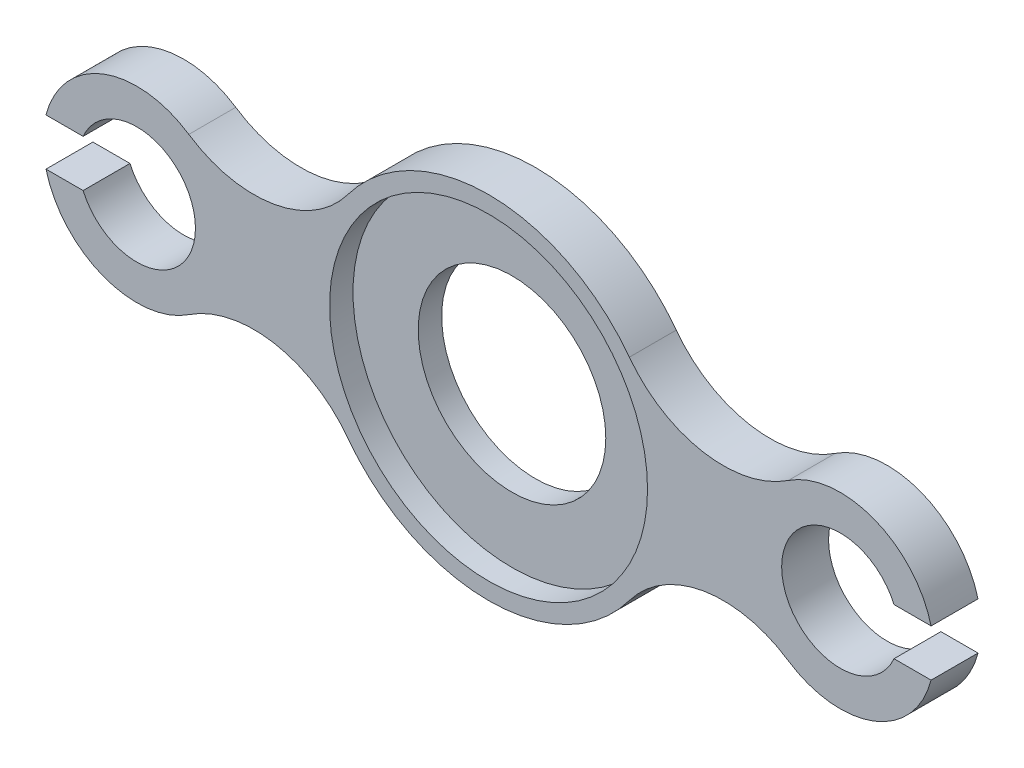
ISO-10303-21;
HEADER;
FILE_DESCRIPTION(('STEP AP214'),'2;1');
FILE_NAME('part.step','',(''),(''),'','','');
FILE_SCHEMA(('AUTOMOTIVE_DESIGN { 1 0 10303 214 1 1 1 1 }'));
ENDSEC;
DATA;
#1=APPLICATION_CONTEXT('core data for automotive mechanical design processes');
#2=APPLICATION_PROTOCOL_DEFINITION('international standard','automotive_design',2000,#1);
#3=PRODUCT_CONTEXT('',#1,'mechanical');
#4=PRODUCT('Part','Part','',(#3));
#5=PRODUCT_RELATED_PRODUCT_CATEGORY('part','',(#4));
#6=PRODUCT_DEFINITION_FORMATION('','',#4);
#7=PRODUCT_DEFINITION_CONTEXT('part definition',#1,'design');
#8=PRODUCT_DEFINITION('design','',#6,#7);
#9=PRODUCT_DEFINITION_SHAPE('','',#8);
#10=(LENGTH_UNIT() NAMED_UNIT(*) SI_UNIT(.MILLI.,.METRE.));
#11=(NAMED_UNIT(*) PLANE_ANGLE_UNIT() SI_UNIT($,.RADIAN.));
#12=(NAMED_UNIT(*) SI_UNIT($,.STERADIAN.) SOLID_ANGLE_UNIT());
#13=UNCERTAINTY_MEASURE_WITH_UNIT(LENGTH_MEASURE(1.E-05),#10,'distance_accuracy_value','');
#14=(GEOMETRIC_REPRESENTATION_CONTEXT(3) GLOBAL_UNCERTAINTY_ASSIGNED_CONTEXT((#13)) GLOBAL_UNIT_ASSIGNED_CONTEXT((#10,
#11,#12)) REPRESENTATION_CONTEXT('',''));
#15=CARTESIAN_POINT('',(0.,0.,0.));
#16=DIRECTION('',(0.,0.,1.));
#17=DIRECTION('',(1.,0.,0.));
#18=AXIS2_PLACEMENT_3D('',#15,#16,#17);
#19=CARTESIAN_POINT('',(0.,0.,20.));
#20=DIRECTION('',(0.,0.,-1.));
#21=DIRECTION('',(-1.,0.,0.));
#22=AXIS2_PLACEMENT_3D('',#19,#20,#21);
#23=CYLINDRICAL_SURFACE('',#22,40.);
#24=CARTESIAN_POINT('',(0.,0.,0.));
#25=DIRECTION('',(0.,0.,1.));
#26=DIRECTION('',(1.,0.,0.));
#27=AXIS2_PLACEMENT_3D('',#24,#25,#26);
#28=CIRCLE('',#27,40.);
#29=CARTESIAN_POINT('',(-38.7298334620742,-10.,0.));
#30=VERTEX_POINT('',#29);
#31=CARTESIAN_POINT('',(22.1851851851852,-33.2838933765123,0.));
#32=VERTEX_POINT('',#31);
#33=EDGE_CURVE('E190',#30,#32,#28,.T.);
#34=ORIENTED_EDGE('',*,*,#33,.T.);
#35=DIRECTION('',(0.,0.,-1.));
#36=VECTOR('',#35,1.);
#37=CARTESIAN_POINT('',(22.1851851851852,-33.2838933765123,20.));
#38=LINE('',#37,#36);
#39=CARTESIAN_POINT('',(22.1851851851852,-33.2838933765123,20.));
#40=VERTEX_POINT('',#39);
#41=EDGE_CURVE('E11',#40,#32,#38,.T.);
#42=ORIENTED_EDGE('',*,*,#41,.F.);
#43=CARTESIAN_POINT('',(0.,0.,20.));
#44=DIRECTION('',(0.,0.,1.));
#45=DIRECTION('',(1.,0.,0.));
#46=AXIS2_PLACEMENT_3D('',#43,#44,#45);
#47=CIRCLE('',#46,40.);
#48=CARTESIAN_POINT('',(-38.7298334620742,-10.,20.));
#49=VERTEX_POINT('',#48);
#50=EDGE_CURVE('E219',#49,#40,#47,.T.);
#51=ORIENTED_EDGE('',*,*,#50,.F.);
#52=DIRECTION('',(0.,0.,-1.));
#53=VECTOR('',#52,1.);
#54=CARTESIAN_POINT('',(-38.7298334620742,-10.,20.));
#55=LINE('',#54,#53);
#56=EDGE_CURVE('E183',#49,#30,#55,.T.);
#57=ORIENTED_EDGE('',*,*,#56,.T.);
#58=EDGE_LOOP('',(#34,#42,#51,#57));
#59=FACE_BOUND('',#58,.T.);
#60=ADVANCED_FACE('F44',(#59),#23,.T.);
#61=CARTESIAN_POINT('',(49.9166666666667,-74.8887600971527,20.));
#62=DIRECTION('',(0.,0.,-1.));
#63=DIRECTION('',(-1.,0.,0.));
#64=AXIS2_PLACEMENT_3D('',#61,#62,#63);
#65=CYLINDRICAL_SURFACE('',#64,50.);
#66=CARTESIAN_POINT('',(49.9166666666667,-74.8887600971527,0.));
#67=DIRECTION('',(0.,0.,-1.));
#68=DIRECTION('',(-1.,0.,0.));
#69=AXIS2_PLACEMENT_3D('',#66,#67,#68);
#70=CIRCLE('',#69,50.);
#71=CARTESIAN_POINT('',(89.95,-44.9332560582916,0.));
#72=VERTEX_POINT('',#71);
#73=EDGE_CURVE('E192',#32,#72,#70,.T.);
#74=ORIENTED_EDGE('',*,*,#73,.T.);
#75=DIRECTION('',(0.,0.,-1.));
#76=VECTOR('',#75,1.);
#77=CARTESIAN_POINT('',(89.95,-44.9332560582916,20.));
#78=LINE('',#77,#76);
#79=CARTESIAN_POINT('',(89.95,-44.9332560582916,20.));
#80=VERTEX_POINT('',#79);
#81=EDGE_CURVE('E52',#80,#72,#78,.T.);
#82=ORIENTED_EDGE('',*,*,#81,.F.);
#83=CARTESIAN_POINT('',(49.9166666666667,-74.8887600971527,20.));
#84=DIRECTION('',(0.,0.,-1.));
#85=DIRECTION('',(-1.,0.,0.));
#86=AXIS2_PLACEMENT_3D('',#83,#84,#85);
#87=CIRCLE('',#86,50.);
#88=EDGE_CURVE('E126',#40,#80,#87,.T.);
#89=ORIENTED_EDGE('',*,*,#88,.F.);
#90=ORIENTED_EDGE('',*,*,#41,.T.);
#91=EDGE_LOOP('',(#74,#82,#89,#90));
#92=FACE_BOUND('',#91,.T.);
#93=ADVANCED_FACE('F319',(#92),#65,.F.);
#94=CARTESIAN_POINT('',(150.,0.,20.));
#95=DIRECTION('',(0.,0.,-1.));
#96=DIRECTION('',(-1.,0.,0.));
#97=AXIS2_PLACEMENT_3D('',#94,#95,#96);
#98=CYLINDRICAL_SURFACE('',#97,75.);
#99=CARTESIAN_POINT('',(150.,0.,0.));
#100=DIRECTION('',(0.,0.,1.));
#101=DIRECTION('',(1.,0.,0.));
#102=AXIS2_PLACEMENT_3D('',#99,#100,#101);
#103=CIRCLE('',#102,75.);
#104=CARTESIAN_POINT('',(210.05,-44.9332560582916,0.));
#105=VERTEX_POINT('',#104);
#106=EDGE_CURVE('E195',#72,#105,#103,.T.);
#107=ORIENTED_EDGE('',*,*,#106,.T.);
#108=DIRECTION('',(0.,0.,-1.));
#109=VECTOR('',#108,1.);
#110=CARTESIAN_POINT('',(210.05,-44.9332560582916,20.));
#111=LINE('',#110,#109);
#112=CARTESIAN_POINT('',(210.05,-44.9332560582916,20.));
#113=VERTEX_POINT('',#112);
#114=EDGE_CURVE('E253',#113,#105,#111,.T.);
#115=ORIENTED_EDGE('',*,*,#114,.F.);
#116=CARTESIAN_POINT('',(150.,0.,20.));
#117=DIRECTION('',(0.,0.,1.));
#118=DIRECTION('',(1.,0.,0.));
#119=AXIS2_PLACEMENT_3D('',#116,#117,#118);
#120=CIRCLE('',#119,75.);
#121=EDGE_CURVE('E259',#80,#113,#120,.T.);
#122=ORIENTED_EDGE('',*,*,#121,.F.);
#123=ORIENTED_EDGE('',*,*,#81,.T.);
#124=EDGE_LOOP('',(#107,#115,#122,#123));
#125=FACE_BOUND('',#124,.T.);
#126=ADVANCED_FACE('F260',(#125),#98,.T.);
#127=CARTESIAN_POINT('',(250.083333333333,-74.8887600971527,20.));
#128=DIRECTION('',(0.,0.,-1.));
#129=DIRECTION('',(-1.,0.,0.));
#130=AXIS2_PLACEMENT_3D('',#127,#128,#129);
#131=CYLINDRICAL_SURFACE('',#130,50.);
#132=CARTESIAN_POINT('',(250.083333333333,-74.8887600971527,0.));
#133=DIRECTION('',(0.,0.,-1.));
#134=DIRECTION('',(-1.,0.,0.));
#135=AXIS2_PLACEMENT_3D('',#132,#133,#134);
#136=CIRCLE('',#135,50.);
#137=CARTESIAN_POINT('',(277.814814814815,-33.2838933765123,0.));
#138=VERTEX_POINT('',#137);
#139=EDGE_CURVE('E197',#105,#138,#136,.T.);
#140=ORIENTED_EDGE('',*,*,#139,.T.);
#141=DIRECTION('',(0.,0.,-1.));
#142=VECTOR('',#141,1.);
#143=CARTESIAN_POINT('',(277.814814814815,-33.2838933765123,20.));
#144=LINE('',#143,#142);
#145=CARTESIAN_POINT('',(277.814814814815,-33.2838933765123,20.));
#146=VERTEX_POINT('',#145);
#147=EDGE_CURVE('E249',#146,#138,#144,.T.);
#148=ORIENTED_EDGE('',*,*,#147,.F.);
#149=CARTESIAN_POINT('',(250.083333333333,-74.8887600971527,20.));
#150=DIRECTION('',(0.,0.,-1.));
#151=DIRECTION('',(-1.,0.,0.));
#152=AXIS2_PLACEMENT_3D('',#149,#150,#151);
#153=CIRCLE('',#152,50.);
#154=EDGE_CURVE('E279',#113,#146,#153,.T.);
#155=ORIENTED_EDGE('',*,*,#154,.F.);
#156=ORIENTED_EDGE('',*,*,#114,.T.);
#157=EDGE_LOOP('',(#140,#148,#155,#156));
#158=FACE_BOUND('',#157,.T.);
#159=ADVANCED_FACE('F267',(#158),#131,.F.);
#160=CARTESIAN_POINT('',(300.,0.,20.));
#161=DIRECTION('',(0.,0.,-1.));
#162=DIRECTION('',(-1.,0.,0.));
#163=AXIS2_PLACEMENT_3D('',#160,#161,#162);
#164=CYLINDRICAL_SURFACE('',#163,40.);
#165=CARTESIAN_POINT('',(300.,0.,0.));
#166=DIRECTION('',(0.,0.,1.));
#167=DIRECTION('',(1.,0.,0.));
#168=AXIS2_PLACEMENT_3D('',#165,#166,#167);
#169=CIRCLE('',#168,40.);
#170=CARTESIAN_POINT('',(338.729833462074,-10.0000000000002,0.));
#171=VERTEX_POINT('',#170);
#172=EDGE_CURVE('E200',#138,#171,#169,.T.);
#173=ORIENTED_EDGE('',*,*,#172,.T.);
#174=DIRECTION('',(0.,0.,-1.));
#175=VECTOR('',#174,1.);
#176=CARTESIAN_POINT('',(338.729833462074,-10.0000000000002,20.));
#177=LINE('',#176,#175);
#178=CARTESIAN_POINT('',(338.729833462074,-10.0000000000002,20.));
#179=VERTEX_POINT('',#178);
#180=EDGE_CURVE('E241',#179,#171,#177,.T.);
#181=ORIENTED_EDGE('',*,*,#180,.F.);
#182=CARTESIAN_POINT('',(300.,0.,20.));
#183=DIRECTION('',(0.,0.,1.));
#184=DIRECTION('',(1.,0.,0.));
#185=AXIS2_PLACEMENT_3D('',#182,#183,#184);
#186=CIRCLE('',#185,40.);
#187=EDGE_CURVE('E274',#146,#179,#186,.T.);
#188=ORIENTED_EDGE('',*,*,#187,.F.);
#189=ORIENTED_EDGE('',*,*,#147,.T.);
#190=EDGE_LOOP('',(#173,#181,#188,#189));
#191=FACE_BOUND('',#190,.T.);
#192=ADVANCED_FACE('F272',(#191),#164,.T.);
#193=CARTESIAN_POINT('',(322.912878474779,-10.0000000000002,20.));
#194=DIRECTION('',(0.,-1.,0.));
#195=DIRECTION('',(0.,0.,-1.));
#196=AXIS2_PLACEMENT_3D('',#193,#194,#195);
#197=PLANE('',#196);
#198=DIRECTION('',(-1.,0.,0.));
#199=VECTOR('',#198,1.);
#200=CARTESIAN_POINT('',(322.912878474779,-10.0000000000002,0.));
#201=LINE('',#200,#199);
#202=CARTESIAN_POINT('',(322.912878474779,-10.0000000000002,0.));
#203=VERTEX_POINT('',#202);
#204=EDGE_CURVE('E203',#171,#203,#201,.T.);
#205=ORIENTED_EDGE('',*,*,#204,.T.);
#206=DIRECTION('',(0.,0.,-1.));
#207=VECTOR('',#206,1.);
#208=CARTESIAN_POINT('',(322.912878474779,-10.0000000000002,20.));
#209=LINE('',#208,#207);
#210=CARTESIAN_POINT('',(322.912878474779,-10.0000000000002,20.));
#211=VERTEX_POINT('',#210);
#212=EDGE_CURVE('E244',#211,#203,#209,.T.);
#213=ORIENTED_EDGE('',*,*,#212,.F.);
#214=DIRECTION('',(-1.,0.,0.));
#215=VECTOR('',#214,1.);
#216=CARTESIAN_POINT('',(322.912878474779,-10.0000000000002,20.));
#217=LINE('',#216,#215);
#218=EDGE_CURVE('E280',#179,#211,#217,.T.);
#219=ORIENTED_EDGE('',*,*,#218,.F.);
#220=ORIENTED_EDGE('',*,*,#180,.T.);
#221=EDGE_LOOP('',(#205,#213,#219,#220));
#222=FACE_BOUND('',#221,.T.);
#223=ADVANCED_FACE('F334',(#222),#197,.F.);
#224=CARTESIAN_POINT('',(300.,0.,20.));
#225=DIRECTION('',(0.,0.,-1.));
#226=DIRECTION('',(-1.,0.,0.));
#227=AXIS2_PLACEMENT_3D('',#224,#225,#226);
#228=CYLINDRICAL_SURFACE('',#227,25.);
#229=CARTESIAN_POINT('',(300.,0.,0.));
#230=DIRECTION('',(0.,0.,-1.));
#231=DIRECTION('',(1.,0.,0.));
#232=AXIS2_PLACEMENT_3D('',#229,#230,#231);
#233=CIRCLE('',#232,25.);
#234=CARTESIAN_POINT('',(322.912878474779,10.0000000000002,0.));
#235=VERTEX_POINT('',#234);
#236=EDGE_CURVE('E201',#203,#235,#233,.T.);
#237=ORIENTED_EDGE('',*,*,#236,.T.);
#238=DIRECTION('',(0.,0.,-1.));
#239=VECTOR('',#238,1.);
#240=CARTESIAN_POINT('',(322.912878474779,10.0000000000002,20.));
#241=LINE('',#240,#239);
#242=CARTESIAN_POINT('',(322.912878474779,10.0000000000002,20.));
#243=VERTEX_POINT('',#242);
#244=EDGE_CURVE('E239',#243,#235,#241,.T.);
#245=ORIENTED_EDGE('',*,*,#244,.F.);
#246=CARTESIAN_POINT('',(300.,0.,20.));
#247=DIRECTION('',(0.,0.,-1.));
#248=DIRECTION('',(1.,0.,0.));
#249=AXIS2_PLACEMENT_3D('',#246,#247,#248);
#250=CIRCLE('',#249,25.);
#251=EDGE_CURVE('E278',#211,#243,#250,.T.);
#252=ORIENTED_EDGE('',*,*,#251,.F.);
#253=ORIENTED_EDGE('',*,*,#212,.T.);
#254=EDGE_LOOP('',(#237,#245,#252,#253));
#255=FACE_BOUND('',#254,.T.);
#256=ADVANCED_FACE('F338',(#255),#228,.F.);
#257=CARTESIAN_POINT('',(338.729833462074,10.0000000000002,20.));
#258=DIRECTION('',(0.,1.,0.));
#259=DIRECTION('',(-1.,0.,0.));
#260=AXIS2_PLACEMENT_3D('',#257,#258,#259);
#261=PLANE('',#260);
#262=DIRECTION('',(1.,0.,0.));
#263=VECTOR('',#262,1.);
#264=CARTESIAN_POINT('',(338.729833462074,10.0000000000002,0.));
#265=LINE('',#264,#263);
#266=CARTESIAN_POINT('',(338.729833462074,10.0000000000002,0.));
#267=VERTEX_POINT('',#266);
#268=EDGE_CURVE('E202',#235,#267,#265,.T.);
#269=ORIENTED_EDGE('',*,*,#268,.T.);
#270=DIRECTION('',(0.,0.,-1.));
#271=VECTOR('',#270,1.);
#272=CARTESIAN_POINT('',(338.729833462074,10.0000000000002,20.));
#273=LINE('',#272,#271);
#274=CARTESIAN_POINT('',(338.729833462074,10.0000000000002,20.));
#275=VERTEX_POINT('',#274);
#276=EDGE_CURVE('E237',#275,#267,#273,.T.);
#277=ORIENTED_EDGE('',*,*,#276,.F.);
#278=DIRECTION('',(1.,0.,0.));
#279=VECTOR('',#278,1.);
#280=CARTESIAN_POINT('',(338.729833462074,10.0000000000002,20.));
#281=LINE('',#280,#279);
#282=EDGE_CURVE('E286',#243,#275,#281,.T.);
#283=ORIENTED_EDGE('',*,*,#282,.F.);
#284=ORIENTED_EDGE('',*,*,#244,.T.);
#285=EDGE_LOOP('',(#269,#277,#283,#284));
#286=FACE_BOUND('',#285,.T.);
#287=ADVANCED_FACE('F336',(#286),#261,.F.);
#288=CARTESIAN_POINT('',(300.,0.,20.));
#289=DIRECTION('',(0.,0.,-1.));
#290=DIRECTION('',(-1.,0.,0.));
#291=AXIS2_PLACEMENT_3D('',#288,#289,#290);
#292=CYLINDRICAL_SURFACE('',#291,40.);
#293=CARTESIAN_POINT('',(300.,0.,0.));
#294=DIRECTION('',(0.,0.,1.));
#295=DIRECTION('',(1.,0.,0.));
#296=AXIS2_PLACEMENT_3D('',#293,#294,#295);
#297=CIRCLE('',#296,40.);
#298=CARTESIAN_POINT('',(277.814814814815,33.2838933765123,0.));
#299=VERTEX_POINT('',#298);
#300=EDGE_CURVE('E210',#267,#299,#297,.T.);
#301=ORIENTED_EDGE('',*,*,#300,.T.);
#302=DIRECTION('',(0.,0.,-1.));
#303=VECTOR('',#302,1.);
#304=CARTESIAN_POINT('',(277.814814814815,33.2838933765123,20.));
#305=LINE('',#304,#303);
#306=CARTESIAN_POINT('',(277.814814814815,33.2838933765123,20.));
#307=VERTEX_POINT('',#306);
#308=EDGE_CURVE('E234',#307,#299,#305,.T.);
#309=ORIENTED_EDGE('',*,*,#308,.F.);
#310=CARTESIAN_POINT('',(300.,0.,20.));
#311=DIRECTION('',(0.,0.,1.));
#312=DIRECTION('',(1.,0.,0.));
#313=AXIS2_PLACEMENT_3D('',#310,#311,#312);
#314=CIRCLE('',#313,40.);
#315=EDGE_CURVE('E289',#275,#307,#314,.T.);
#316=ORIENTED_EDGE('',*,*,#315,.F.);
#317=ORIENTED_EDGE('',*,*,#276,.T.);
#318=EDGE_LOOP('',(#301,#309,#316,#317));
#319=FACE_BOUND('',#318,.T.);
#320=ADVANCED_FACE('F343',(#319),#292,.T.);
#321=CARTESIAN_POINT('',(250.083333333333,74.8887600971527,20.));
#322=DIRECTION('',(0.,0.,-1.));
#323=DIRECTION('',(-1.,0.,0.));
#324=AXIS2_PLACEMENT_3D('',#321,#322,#323);
#325=CYLINDRICAL_SURFACE('',#324,50.);
#326=CARTESIAN_POINT('',(250.083333333333,74.8887600971527,0.));
#327=DIRECTION('',(0.,0.,-1.));
#328=DIRECTION('',(1.,0.,0.));
#329=AXIS2_PLACEMENT_3D('',#326,#327,#328);
#330=CIRCLE('',#329,50.);
#331=CARTESIAN_POINT('',(210.05,44.9332560582916,0.));
#332=VERTEX_POINT('',#331);
#333=EDGE_CURVE('E207',#299,#332,#330,.T.);
#334=ORIENTED_EDGE('',*,*,#333,.T.);
#335=DIRECTION('',(0.,0.,-1.));
#336=VECTOR('',#335,1.);
#337=CARTESIAN_POINT('',(210.05,44.9332560582916,20.));
#338=LINE('',#337,#336);
#339=CARTESIAN_POINT('',(210.05,44.9332560582916,20.));
#340=VERTEX_POINT('',#339);
#341=EDGE_CURVE('E226',#340,#332,#338,.T.);
#342=ORIENTED_EDGE('',*,*,#341,.F.);
#343=CARTESIAN_POINT('',(250.083333333333,74.8887600971527,20.));
#344=DIRECTION('',(0.,0.,-1.));
#345=DIRECTION('',(1.,0.,0.));
#346=AXIS2_PLACEMENT_3D('',#343,#344,#345);
#347=CIRCLE('',#346,50.);
#348=EDGE_CURVE('E290',#307,#340,#347,.T.);
#349=ORIENTED_EDGE('',*,*,#348,.F.);
#350=ORIENTED_EDGE('',*,*,#308,.T.);
#351=EDGE_LOOP('',(#334,#342,#349,#350));
#352=FACE_BOUND('',#351,.T.);
#353=ADVANCED_FACE('F346',(#352),#325,.F.);
#354=CARTESIAN_POINT('',(150.,0.,20.));
#355=DIRECTION('',(0.,0.,-1.));
#356=DIRECTION('',(-1.,0.,0.));
#357=AXIS2_PLACEMENT_3D('',#354,#355,#356);
#358=CYLINDRICAL_SURFACE('',#357,75.);
#359=CARTESIAN_POINT('',(150.,0.,0.));
#360=DIRECTION('',(0.,0.,1.));
#361=DIRECTION('',(1.,0.,0.));
#362=AXIS2_PLACEMENT_3D('',#359,#360,#361);
#363=CIRCLE('',#362,75.);
#364=CARTESIAN_POINT('',(89.95,44.9332560582916,0.));
#365=VERTEX_POINT('',#364);
#366=EDGE_CURVE('E211',#332,#365,#363,.T.);
#367=ORIENTED_EDGE('',*,*,#366,.T.);
#368=DIRECTION('',(0.,0.,-1.));
#369=VECTOR('',#368,1.);
#370=CARTESIAN_POINT('',(89.95,44.9332560582916,20.));
#371=LINE('',#370,#369);
#372=CARTESIAN_POINT('',(89.95,44.9332560582916,20.));
#373=VERTEX_POINT('',#372);
#374=EDGE_CURVE('E229',#373,#365,#371,.T.);
#375=ORIENTED_EDGE('',*,*,#374,.F.);
#376=CARTESIAN_POINT('',(150.,0.,20.));
#377=DIRECTION('',(0.,0.,1.));
#378=DIRECTION('',(1.,0.,0.));
#379=AXIS2_PLACEMENT_3D('',#376,#377,#378);
#380=CIRCLE('',#379,75.);
#381=EDGE_CURVE('E295',#340,#373,#380,.T.);
#382=ORIENTED_EDGE('',*,*,#381,.F.);
#383=ORIENTED_EDGE('',*,*,#341,.T.);
#384=EDGE_LOOP('',(#367,#375,#382,#383));
#385=FACE_BOUND('',#384,.T.);
#386=ADVANCED_FACE('F354',(#385),#358,.T.);
#387=CARTESIAN_POINT('',(49.9166666666667,74.8887600971527,20.));
#388=DIRECTION('',(0.,0.,-1.));
#389=DIRECTION('',(-1.,0.,0.));
#390=AXIS2_PLACEMENT_3D('',#387,#388,#389);
#391=CYLINDRICAL_SURFACE('',#390,50.);
#392=CARTESIAN_POINT('',(49.9166666666667,74.8887600971527,0.));
#393=DIRECTION('',(0.,0.,-1.));
#394=DIRECTION('',(1.,0.,0.));
#395=AXIS2_PLACEMENT_3D('',#392,#393,#394);
#396=CIRCLE('',#395,50.);
#397=CARTESIAN_POINT('',(22.1851851851852,33.2838933765123,0.));
#398=VERTEX_POINT('',#397);
#399=EDGE_CURVE('E213',#365,#398,#396,.T.);
#400=ORIENTED_EDGE('',*,*,#399,.T.);
#401=DIRECTION('',(0.,0.,-1.));
#402=VECTOR('',#401,1.);
#403=CARTESIAN_POINT('',(22.1851851851852,33.2838933765123,20.));
#404=LINE('',#403,#402);
#405=CARTESIAN_POINT('',(22.1851851851852,33.2838933765123,20.));
#406=VERTEX_POINT('',#405);
#407=EDGE_CURVE('E221',#406,#398,#404,.T.);
#408=ORIENTED_EDGE('',*,*,#407,.F.);
#409=CARTESIAN_POINT('',(49.9166666666667,74.8887600971527,20.));
#410=DIRECTION('',(0.,0.,-1.));
#411=DIRECTION('',(1.,0.,0.));
#412=AXIS2_PLACEMENT_3D('',#409,#410,#411);
#413=CIRCLE('',#412,50.);
#414=EDGE_CURVE('E294',#373,#406,#413,.T.);
#415=ORIENTED_EDGE('',*,*,#414,.F.);
#416=ORIENTED_EDGE('',*,*,#374,.T.);
#417=EDGE_LOOP('',(#400,#408,#415,#416));
#418=FACE_BOUND('',#417,.T.);
#419=ADVANCED_FACE('F296',(#418),#391,.F.);
#420=CARTESIAN_POINT('',(0.,0.,20.));
#421=DIRECTION('',(0.,0.,-1.));
#422=DIRECTION('',(-1.,0.,0.));
#423=AXIS2_PLACEMENT_3D('',#420,#421,#422);
#424=CYLINDRICAL_SURFACE('',#423,40.);
#425=CARTESIAN_POINT('',(0.,0.,0.));
#426=DIRECTION('',(0.,0.,1.));
#427=DIRECTION('',(1.,0.,0.));
#428=AXIS2_PLACEMENT_3D('',#425,#426,#427);
#429=CIRCLE('',#428,40.);
#430=CARTESIAN_POINT('',(-38.7298334620742,10.,0.));
#431=VERTEX_POINT('',#430);
#432=EDGE_CURVE('E214',#398,#431,#429,.T.);
#433=ORIENTED_EDGE('',*,*,#432,.T.);
#434=DIRECTION('',(0.,0.,-1.));
#435=VECTOR('',#434,1.);
#436=CARTESIAN_POINT('',(-38.7298334620742,10.,20.));
#437=LINE('',#436,#435);
#438=CARTESIAN_POINT('',(-38.7298334620742,10.,20.));
#439=VERTEX_POINT('',#438);
#440=EDGE_CURVE('E180',#439,#431,#437,.T.);
#441=ORIENTED_EDGE('',*,*,#440,.F.);
#442=CARTESIAN_POINT('',(0.,0.,20.));
#443=DIRECTION('',(0.,0.,1.));
#444=DIRECTION('',(1.,0.,0.));
#445=AXIS2_PLACEMENT_3D('',#442,#443,#444);
#446=CIRCLE('',#445,40.);
#447=EDGE_CURVE('E173',#406,#439,#446,.T.);
#448=ORIENTED_EDGE('',*,*,#447,.F.);
#449=ORIENTED_EDGE('',*,*,#407,.T.);
#450=EDGE_LOOP('',(#433,#441,#448,#449));
#451=FACE_BOUND('',#450,.T.);
#452=ADVANCED_FACE('F303',(#451),#424,.T.);
#453=CARTESIAN_POINT('',(-38.7298334620742,10.,20.));
#454=DIRECTION('',(0.,1.,0.));
#455=DIRECTION('',(0.,0.,1.));
#456=AXIS2_PLACEMENT_3D('',#453,#454,#455);
#457=PLANE('',#456);
#458=DIRECTION('',(1.,0.,0.));
#459=VECTOR('',#458,1.);
#460=CARTESIAN_POINT('',(-38.7298334620742,10.,0.));
#461=LINE('',#460,#459);
#462=CARTESIAN_POINT('',(-22.9128784747792,10.,0.));
#463=VERTEX_POINT('',#462);
#464=EDGE_CURVE('E178',#431,#463,#461,.T.);
#465=ORIENTED_EDGE('',*,*,#464,.T.);
#466=DIRECTION('',(0.,0.,-1.));
#467=VECTOR('',#466,1.);
#468=CARTESIAN_POINT('',(-22.9128784747792,10.,20.));
#469=LINE('',#468,#467);
#470=CARTESIAN_POINT('',(-22.9128784747792,10.,20.));
#471=VERTEX_POINT('',#470);
#472=EDGE_CURVE('E176',#471,#463,#469,.T.);
#473=ORIENTED_EDGE('',*,*,#472,.F.);
#474=DIRECTION('',(1.,0.,0.));
#475=VECTOR('',#474,1.);
#476=CARTESIAN_POINT('',(-38.7298334620742,10.,20.));
#477=LINE('',#476,#475);
#478=EDGE_CURVE('E164',#439,#471,#477,.T.);
#479=ORIENTED_EDGE('',*,*,#478,.F.);
#480=ORIENTED_EDGE('',*,*,#440,.T.);
#481=EDGE_LOOP('',(#465,#473,#479,#480));
#482=FACE_BOUND('',#481,.T.);
#483=ADVANCED_FACE('F177',(#482),#457,.F.);
#484=CARTESIAN_POINT('',(0.,0.,20.));
#485=DIRECTION('',(0.,0.,-1.));
#486=DIRECTION('',(-1.,0.,0.));
#487=AXIS2_PLACEMENT_3D('',#484,#485,#486);
#488=CYLINDRICAL_SURFACE('',#487,25.);
#489=CARTESIAN_POINT('',(0.,0.,0.));
#490=DIRECTION('',(0.,0.,-1.));
#491=DIRECTION('',(1.,0.,0.));
#492=AXIS2_PLACEMENT_3D('',#489,#490,#491);
#493=CIRCLE('',#492,25.);
#494=CARTESIAN_POINT('',(-22.9128784747792,-10.,0.));
#495=VERTEX_POINT('',#494);
#496=EDGE_CURVE('E111',#463,#495,#493,.T.);
#497=ORIENTED_EDGE('',*,*,#496,.T.);
#498=DIRECTION('',(0.,0.,-1.));
#499=VECTOR('',#498,1.);
#500=CARTESIAN_POINT('',(-22.9128784747792,-10.,20.));
#501=LINE('',#500,#499);
#502=CARTESIAN_POINT('',(-22.9128784747792,-10.,20.));
#503=VERTEX_POINT('',#502);
#504=EDGE_CURVE('E182',#503,#495,#501,.T.);
#505=ORIENTED_EDGE('',*,*,#504,.F.);
#506=CARTESIAN_POINT('',(0.,0.,20.));
#507=DIRECTION('',(0.,0.,-1.));
#508=DIRECTION('',(1.,0.,0.));
#509=AXIS2_PLACEMENT_3D('',#506,#507,#508);
#510=CIRCLE('',#509,25.);
#511=EDGE_CURVE('E166',#471,#503,#510,.T.);
#512=ORIENTED_EDGE('',*,*,#511,.F.);
#513=ORIENTED_EDGE('',*,*,#472,.T.);
#514=EDGE_LOOP('',(#497,#505,#512,#513));
#515=FACE_BOUND('',#514,.T.);
#516=ADVANCED_FACE('F181',(#515),#488,.F.);
#517=CARTESIAN_POINT('',(-38.7298334620742,-10.,20.));
#518=DIRECTION('',(0.,-1.,0.));
#519=DIRECTION('',(0.,0.,-1.));
#520=AXIS2_PLACEMENT_3D('',#517,#518,#519);
#521=PLANE('',#520);
#522=DIRECTION('',(-1.,0.,0.));
#523=VECTOR('',#522,1.);
#524=CARTESIAN_POINT('',(-38.7298334620742,-10.,0.));
#525=LINE('',#524,#523);
#526=EDGE_CURVE('E116',#495,#30,#525,.T.);
#527=ORIENTED_EDGE('',*,*,#526,.T.);
#528=ORIENTED_EDGE('',*,*,#56,.F.);
#529=DIRECTION('',(-1.,0.,0.));
#530=VECTOR('',#529,1.);
#531=CARTESIAN_POINT('',(-38.7298334620742,-10.,20.));
#532=LINE('',#531,#530);
#533=EDGE_CURVE('E63',#503,#49,#532,.T.);
#534=ORIENTED_EDGE('',*,*,#533,.F.);
#535=ORIENTED_EDGE('',*,*,#504,.T.);
#536=EDGE_LOOP('',(#527,#528,#534,#535));
#537=FACE_BOUND('',#536,.T.);
#538=ADVANCED_FACE('F306',(#537),#521,.F.);
#539=CARTESIAN_POINT('',(0.,0.,20.));
#540=DIRECTION('',(0.,0.,1.));
#541=DIRECTION('',(1.,0.,0.));
#542=AXIS2_PLACEMENT_3D('',#539,#540,#541);
#543=PLANE('',#542);
#544=CARTESIAN_POINT('',(150.,0.,20.));
#545=DIRECTION('',(0.,0.,1.));
#546=DIRECTION('',(1.,0.,0.));
#547=AXIS2_PLACEMENT_3D('',#544,#545,#546);
#548=CIRCLE('',#547,67.8);
#549=CARTESIAN_POINT('',(217.8,0.,20.));
#550=VERTEX_POINT('',#549);
#551=EDGE_CURVE('E194',#550,#550,#548,.T.);
#552=ORIENTED_EDGE('',*,*,#551,.F.);
#553=EDGE_LOOP('',(#552));
#554=FACE_BOUND('',#553,.T.);
#555=ORIENTED_EDGE('',*,*,#50,.T.);
#556=ORIENTED_EDGE('',*,*,#88,.T.);
#557=ORIENTED_EDGE('',*,*,#121,.T.);
#558=ORIENTED_EDGE('',*,*,#154,.T.);
#559=ORIENTED_EDGE('',*,*,#187,.T.);
#560=ORIENTED_EDGE('',*,*,#218,.T.);
#561=ORIENTED_EDGE('',*,*,#251,.T.);
#562=ORIENTED_EDGE('',*,*,#282,.T.);
#563=ORIENTED_EDGE('',*,*,#315,.T.);
#564=ORIENTED_EDGE('',*,*,#348,.T.);
#565=ORIENTED_EDGE('',*,*,#381,.T.);
#566=ORIENTED_EDGE('',*,*,#414,.T.);
#567=ORIENTED_EDGE('',*,*,#447,.T.);
#568=ORIENTED_EDGE('',*,*,#478,.T.);
#569=ORIENTED_EDGE('',*,*,#511,.T.);
#570=ORIENTED_EDGE('',*,*,#533,.T.);
#571=EDGE_LOOP('',(#555,#556,#557,#558,#559,#560,#561,#562,#563,#564,#565,#566,#567,#568,#569,#570));
#572=FACE_BOUND('',#571,.T.);
#573=ADVANCED_FACE('F170',(#554,#572),#543,.T.);
#574=CARTESIAN_POINT('',(0.,0.,0.));
#575=DIRECTION('',(0.,0.,1.));
#576=DIRECTION('',(1.,0.,0.));
#577=AXIS2_PLACEMENT_3D('',#574,#575,#576);
#578=PLANE('',#577);
#579=ORIENTED_EDGE('',*,*,#33,.F.);
#580=ORIENTED_EDGE('',*,*,#526,.F.);
#581=ORIENTED_EDGE('',*,*,#496,.F.);
#582=ORIENTED_EDGE('',*,*,#464,.F.);
#583=ORIENTED_EDGE('',*,*,#432,.F.);
#584=ORIENTED_EDGE('',*,*,#399,.F.);
#585=ORIENTED_EDGE('',*,*,#366,.F.);
#586=ORIENTED_EDGE('',*,*,#333,.F.);
#587=ORIENTED_EDGE('',*,*,#300,.F.);
#588=ORIENTED_EDGE('',*,*,#268,.F.);
#589=ORIENTED_EDGE('',*,*,#236,.F.);
#590=ORIENTED_EDGE('',*,*,#204,.F.);
#591=ORIENTED_EDGE('',*,*,#172,.F.);
#592=ORIENTED_EDGE('',*,*,#139,.F.);
#593=ORIENTED_EDGE('',*,*,#106,.F.);
#594=ORIENTED_EDGE('',*,*,#73,.F.);
#595=EDGE_LOOP('',(#579,#580,#581,#582,#583,#584,#585,#586,#587,#588,#589,#590,#591,#592,#593,#594));
#596=FACE_BOUND('',#595,.T.);
#597=CARTESIAN_POINT('',(150.,0.,0.));
#598=DIRECTION('',(0.,0.,1.));
#599=DIRECTION('',(1.,0.,0.));
#600=AXIS2_PLACEMENT_3D('',#597,#598,#599);
#601=CIRCLE('',#600,40.);
#602=CARTESIAN_POINT('',(190.,0.,0.));
#603=VERTEX_POINT('',#602);
#604=EDGE_CURVE('E618',#603,#603,#601,.T.);
#605=ORIENTED_EDGE('',*,*,#604,.T.);
#606=EDGE_LOOP('',(#605));
#607=FACE_BOUND('',#606,.T.);
#608=ADVANCED_FACE('F263',(#596,#607),#578,.F.);
#609=CARTESIAN_POINT('',(150.,0.,0.));
#610=DIRECTION('',(0.,0.,1.));
#611=DIRECTION('',(1.,0.,0.));
#612=AXIS2_PLACEMENT_3D('',#609,#610,#611);
#613=CYLINDRICAL_SURFACE('',#612,67.8);
#614=CARTESIAN_POINT('',(150.,0.,10.));
#615=DIRECTION('',(0.,0.,1.));
#616=DIRECTION('',(1.,0.,0.));
#617=AXIS2_PLACEMENT_3D('',#614,#615,#616);
#618=CIRCLE('',#617,67.8);
#619=CARTESIAN_POINT('',(217.8,0.,10.));
#620=VERTEX_POINT('',#619);
#621=EDGE_CURVE('E611',#620,#620,#618,.T.);
#622=ORIENTED_EDGE('',*,*,#621,.F.);
#623=EDGE_LOOP('',(#622));
#624=FACE_BOUND('',#623,.T.);
#625=ORIENTED_EDGE('',*,*,#551,.T.);
#626=EDGE_LOOP('',(#625));
#627=FACE_BOUND('',#626,.T.);
#628=ADVANCED_FACE('F392',(#624,#627),#613,.F.);
#629=CARTESIAN_POINT('',(150.,0.,10.));
#630=DIRECTION('',(0.,0.,1.));
#631=DIRECTION('',(1.,0.,0.));
#632=AXIS2_PLACEMENT_3D('',#629,#630,#631);
#633=PLANE('',#632);
#634=CARTESIAN_POINT('',(150.,0.,10.));
#635=DIRECTION('',(0.,0.,1.));
#636=DIRECTION('',(1.,0.,0.));
#637=AXIS2_PLACEMENT_3D('',#634,#635,#636);
#638=CIRCLE('',#637,40.);
#639=CARTESIAN_POINT('',(190.,0.,10.));
#640=VERTEX_POINT('',#639);
#641=EDGE_CURVE('E624',#640,#640,#638,.T.);
#642=ORIENTED_EDGE('',*,*,#641,.F.);
#643=EDGE_LOOP('',(#642));
#644=FACE_BOUND('',#643,.T.);
#645=ORIENTED_EDGE('',*,*,#621,.T.);
#646=EDGE_LOOP('',(#645));
#647=FACE_BOUND('',#646,.T.);
#648=ADVANCED_FACE('F398',(#644,#647),#633,.T.);
#649=CARTESIAN_POINT('',(150.,0.,0.));
#650=DIRECTION('',(0.,0.,1.));
#651=DIRECTION('',(1.,0.,0.));
#652=AXIS2_PLACEMENT_3D('',#649,#650,#651);
#653=CYLINDRICAL_SURFACE('',#652,40.);
#654=ORIENTED_EDGE('',*,*,#604,.F.);
#655=EDGE_LOOP('',(#654));
#656=FACE_BOUND('',#655,.T.);
#657=ORIENTED_EDGE('',*,*,#641,.T.);
#658=EDGE_LOOP('',(#657));
#659=FACE_BOUND('',#658,.T.);
#660=ADVANCED_FACE('F402',(#656,#659),#653,.F.);
#661=CLOSED_SHELL('',(#60,#93,#126,#159,#192,#223,#256,#287,#320,#353,#386,#419,#452,#483,#516,
#538,#573,#608,#628,#648,#660));
#662=MANIFOLD_SOLID_BREP('B2',#661);
#663=ADVANCED_BREP_SHAPE_REPRESENTATION('',(#18,#662),#14);
#664=SHAPE_DEFINITION_REPRESENTATION(#9,#663);
ENDSEC;
END-ISO-10303-21;
